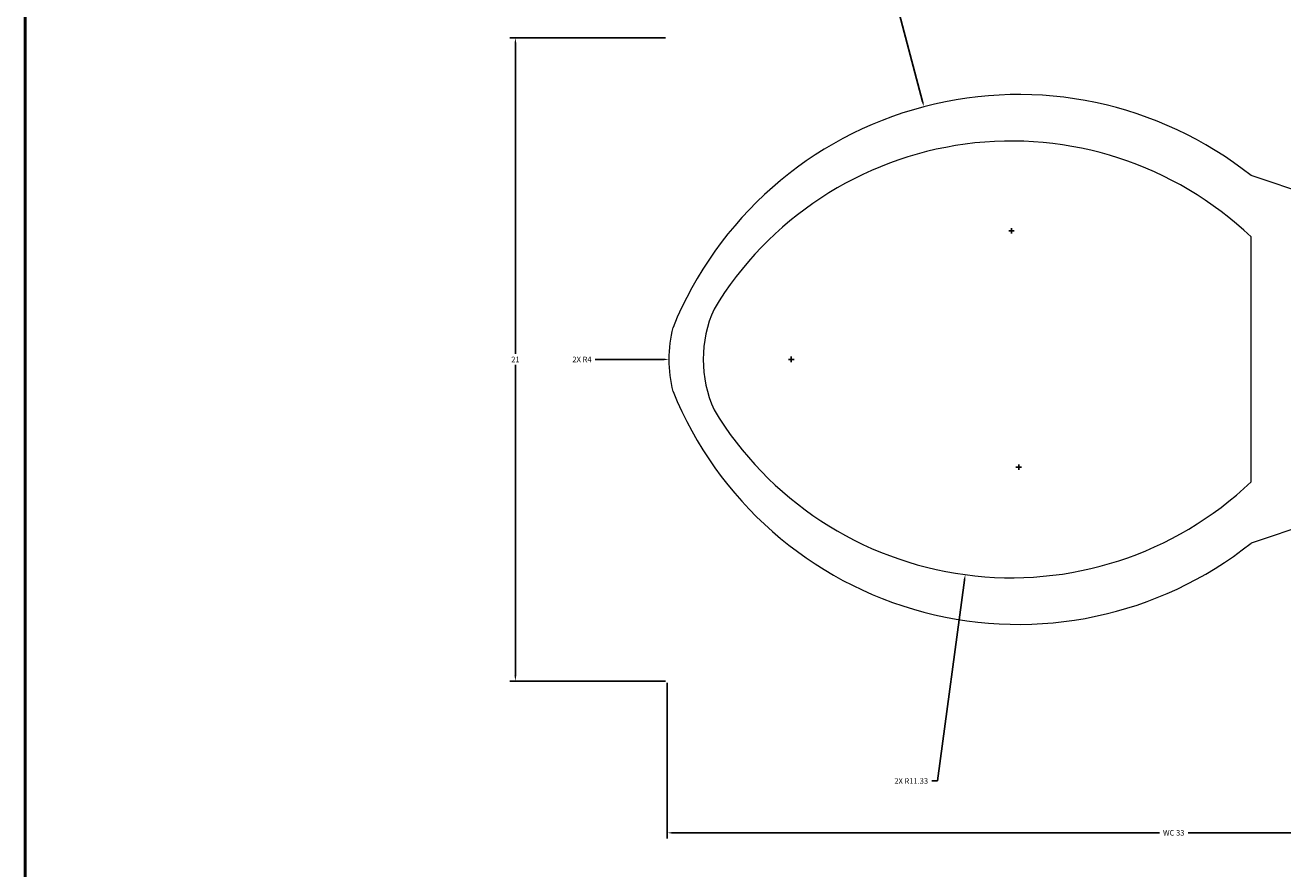
# Model space of a CAD drawing. Units: inches. Extents: x 2621 to 2849, y 2066 to 2463.
# Tile 25 of 28: x 2768 to 2809, y 2407 to 2435. Entities that reach past the tile are written whole.
import ezdxf

# ---------------------------------------------------------------- set-up
doc = ezdxf.new("R2010")
doc.units = ezdxf.units.IN
for name, color, linetype, lineweight in [('A-ANNO-DIMS', 2, 'Continuous', 18), ('A-FLOR-FIXT', 9, 'Continuous', 18), ('A-WALL', 7, 'Continuous', 50)]:
    doc.layers.add(name, color=color, linetype=linetype, lineweight=lineweight)
doc.styles.get("Standard").update_dxf_attribs({"font": 'arial.ttf'})
doc.dimstyles.get("Standard").update_dxf_attribs({"dimtxt": 0.18, "dimasz": 0.18, "dimexe": 0.18, "dimexo": 0.0625, "dimgap": 0.09, "dimtad": 0, "dimtih": 1, "dimtoh": 1, "dimdec": 4, "dimzin": 0, "dimdsep": 46, "dimtxsty": 'Standard', "dimcen": 0.09, "dimadec": 0, "dimazin": 0, "dimtfac": 1, "dimtdec": 4, "dimtofl": 0, "dimtmove": 0, "dimatfit": 3, "dimfxl": 1, "dimtolj": 1, "dimtzin": 0, "dimarcsym": 0})

# ---------------------------------------------------------------- blocks, each defined once
blk = doc.blocks.new('Toilet - top')
for p, q in [((9.5, -6), (9.5, -2)), ((-8, -8.5), (-8, -8)), ((-7, -8), (-7, -9.5)), ((-4, -8), (-6, -14)), ((4, -8), (6, -14)), ((-10, -8.5), (-8, -8.5)), ((-10, -9.5), (-10, -8.5)), ((-7, -9.5), (-10, -9.5)), ((4, -14), (-4, -14))]:
    blk.add_line(p, q)
blk.add_lwpolyline([(10.5, -8), (10.5, 0), (-10.5, 0), (-10.5, -8)], close=True)
for points in [[(8.5, -1), (-8.5, -1)], [(-9.5, -2), (-9.5, -6)], [(-8.5, -7), (8.5, -7)]]:
    blk.add_lwpolyline(points)
for centre, radius, start, end in [((-8.625, -1.875), 0.884, 81.8699, 188.1301), ((8.625, -1.875), 0.884, 351.8699, 98.1301), ((-8.625, -6.125), 0.884, 171.8699, 278.1301), ((8.625, -6.125), 0.884, 261.8699, 8.1301), ((3.52, -21.58), 12.169, 141.4691, 247.9714), ((4.2, -21.817), 11.329, 136.3677, 238.9468), ((-3.519, -21.58), 12.169, 292.0284, 38.5307), ((-4.2, -21.817), 11.329, 301.053, 43.6321), ((0, -27.876), 4, 245.7318, 294.2682), ((0, -29), 4, 254.8605, 285.1395)]:
    blk.add_arc(centre, radius, start, end)
blk = doc.blocks.new('*D27')
at = {"layer": 'A-ANNO-DIMS', "color": 0, "lineweight": -2, "transparency": 16777216}
for p, q in [((2788.824, 2413.484), (2788.824, 2408.409)), ((2821.87, 2413.484), (2821.87, 2408.409)), ((2789.004, 2408.589), (2804.88, 2408.589)), ((2821.69, 2408.589), (2805.814, 2408.589))]:
    blk.add_line(p, q, dxfattribs=at)
at = {"layer": 'A-ANNO-DIMS', "color": 0, "transparency": 16777216}
for points in [[(2789.004, 2408.619), (2789.004, 2408.559), (2788.824, 2408.589)], [(2821.69, 2408.619), (2821.69, 2408.559), (2821.87, 2408.589)]]:
    blk.add_solid(points, dxfattribs=at)
at = {"layer": 'Defpoints', "color": 0, "transparency": 16777216}
for p in [(2788.824, 2413.546), (2821.87, 2413.546), (2821.87, 2408.589)]:
    blk.add_point(p, dxfattribs=at)
at = {"layer": 'A-ANNO-DIMS', "color": 0, "transparency": 16777216, "insert": (2805.347, 2408.589), "char_height": 0.18, "attachment_point": 5}
blk.add_mtext('\\A1;WC 33', dxfattribs=at)
blk = doc.blocks.new('*D28')
at = {"layer": 'A-ANNO-DIMS', "color": 0, "lineweight": -2, "transparency": 16777216}
for p, q in [((2788.761, 2434.546), (2783.687, 2434.546)), ((2783.867, 2434.366), (2783.867, 2424.226)), ((2783.867, 2413.726), (2783.867, 2423.866)), ((2788.761, 2413.546), (2783.687, 2413.546))]:
    blk.add_line(p, q, dxfattribs=at)
at = {"layer": 'A-ANNO-DIMS', "color": 0, "transparency": 16777216}
for points in [[(2783.837, 2434.366), (2783.897, 2434.366), (2783.867, 2434.546)], [(2783.837, 2413.726), (2783.897, 2413.726), (2783.867, 2413.546)]]:
    blk.add_solid(points, dxfattribs=at)
at = {"layer": 'Defpoints', "color": 0, "transparency": 16777216}
for p in [(2788.824, 2434.546), (2783.867, 2413.546), (2788.824, 2413.546)]:
    blk.add_point(p, dxfattribs=at)
at = {"layer": 'A-ANNO-DIMS', "color": 0, "transparency": 16777216, "insert": (2783.867, 2424.046), "char_height": 0.18, "attachment_point": 5}
blk.add_mtext('\\A1;21', dxfattribs=at)
blk = doc.blocks.new('*D71')
at = {"layer": 'A-ANNO-DIMS', "color": 0, "lineweight": -2, "transparency": 16777216}
for p, q in [((2795.161, 2439.358), (2795.341, 2439.358)), ((2795.341, 2439.358), (2797.151, 2432.47)), ((2800.2, 2420.527), (2800.38, 2420.527)), ((2800.29, 2420.437), (2800.29, 2420.617))]:
    blk.add_line(p, q, dxfattribs=at)
at = {"layer": 'A-ANNO-DIMS', "color": 0, "transparency": 16777216}
blk.add_solid([(2797.18, 2432.478), (2797.122, 2432.463), (2797.197, 2432.296)], dxfattribs=at)
at = {"layer": 'Defpoints', "color": 0, "transparency": 16777216}
for p in [(2797.197, 2432.296), (2800.29, 2420.527)]:
    blk.add_point(p, dxfattribs=at)
at = {"layer": 'A-ANNO-DIMS', "color": 0, "transparency": 16777216, "insert": (2794.487, 2439.358), "char_height": 0.18, "attachment_point": 5}
blk.add_mtext('\\A1;2X R12.17', dxfattribs=at)
blk = doc.blocks.new('*D72')
at = {"layer": 'A-ANNO-DIMS', "color": 0, "lineweight": -2, "transparency": 16777216}
for p, q in [((2799.963, 2428.246), (2800.143, 2428.246)), ((2800.053, 2428.156), (2800.053, 2428.336)), ((2797.637, 2410.281), (2798.519, 2416.839)), ((2797.457, 2410.281), (2797.637, 2410.281))]:
    blk.add_line(p, q, dxfattribs=at)
at = {"layer": 'A-ANNO-DIMS', "color": 0, "transparency": 16777216}
blk.add_solid([(2798.489, 2416.843), (2798.549, 2416.835), (2798.543, 2417.018)], dxfattribs=at)
at = {"layer": 'Defpoints', "color": 0, "transparency": 16777216}
for p in [(2800.053, 2428.246), (2798.543, 2417.018)]:
    blk.add_point(p, dxfattribs=at)
at = {"layer": 'A-ANNO-DIMS', "color": 0, "transparency": 16777216, "insert": (2796.782, 2410.281), "char_height": 0.18, "attachment_point": 5}
blk.add_mtext('\\A1;2X R11.33', dxfattribs=at)
blk = doc.blocks.new('*D74')
at = {"layer": 'A-ANNO-DIMS', "color": 0, "lineweight": -2, "transparency": 16777216}
for p, q in [((2792.87, 2423.956), (2792.87, 2424.136)), ((2786.47, 2424.046), (2788.69, 2424.046)), ((2792.78, 2424.046), (2792.96, 2424.046))]:
    blk.add_line(p, q, dxfattribs=at)
at = {"layer": 'A-ANNO-DIMS', "color": 0, "transparency": 16777216}
blk.add_solid([(2788.69, 2424.076), (2788.69, 2424.016), (2788.87, 2424.046)], dxfattribs=at)
at = {"layer": 'Defpoints', "color": 0, "transparency": 16777216}
for p in [(2788.87, 2424.046), (2792.87, 2424.046)]:
    blk.add_point(p, dxfattribs=at)
at = {"layer": 'A-ANNO-DIMS', "color": 0, "transparency": 16777216, "insert": (2786.04, 2424.046), "char_height": 0.18, "attachment_point": 5}
blk.add_mtext('\\A1;2X R4', dxfattribs=at)

msp = doc.modelspace()

# ---------------------------------------------------------------- linework, layer by layer
at = {"layer": 'A-WALL'}
msp.add_line((2767.8701, 2375.3746), (2767.8701, 2435.3746), dxfattribs=at)

# ---------------------------------------------------------------- block references
at = {"layer": 'A-FLOR-FIXT', "rotation": 270}
msp.add_blockref('Toilet - top', (2821.8701, 2424.0461), dxfattribs=at)

# ---------------------------------------------------------------- dimensions: what is measured, and where the dimension line sits
at = {"layer": 'A-ANNO-DIMS'}
for center, mpoint, override, picture, middle in [((2800.2896, 2420.5266), (2797.197, 2432.296), {"dimdec": 2, "dimlfac": 1, "dimrnd": 0, "dimzin": 0, "dimdsep": 46, "dimlunit": 2}, '*D71', (2794.4867, 2439.3577)), ((2800.0527, 2428.246), (2798.543, 2417.0179), {"dimdec": 2, "dimlfac": 1, "dimrnd": 0, "dimzin": 0, "dimdsep": 46, "dimlunit": 2}, '*D72', (2796.7824, 2410.281)), ((2792.8701, 2424.0461), (2788.8701, 2424.046), {"dimdec": 0, "dimlfac": 1, "dimrnd": 0, "dimzin": 0, "dimdsep": 46, "dimlunit": 2}, '*D74', (2786.4701, 2424.0459))]:
    dim = msp.add_radius_dim(center=center, mpoint=mpoint, text='2X <>', dimstyle='Standard', override=override, dxfattribs=at)
    dim.commit()
    dim.dimension.update_dxf_attribs({"geometry": picture, "text_midpoint": middle, "dimtype": 164})
dim = msp.add_linear_dim(base=(2783.8669, 2413.5461), p1=(2788.8239, 2434.5461), p2=(2788.8239, 2413.5461), angle=270, dimstyle='Standard', override={"dimdec": 0, "dimlfac": 1, "dimrnd": 0, "dimzin": 0, "dimdsep": 46, "dimlunit": 2}, dxfattribs=at)
dim.commit()
dim.dimension.update_dxf_attribs({"geometry": '*D28', "text_midpoint": (2783.8669, 2424.0461)})
dim = msp.add_linear_dim(base=(2821.8701, 2408.5892), p1=(2788.8239, 2413.5461), p2=(2821.8701, 2413.5461), text='WC <>', dimstyle='Standard', override={"dimdec": 0, "dimlfac": 1, "dimrnd": 0, "dimzin": 0, "dimdsep": 46, "dimlunit": 2}, dxfattribs=at)
dim.commit()
dim.dimension.update_dxf_attribs({"geometry": '*D27', "text_midpoint": (2805.347, 2408.5892)})

doc.saveas('drawing.dxf')
